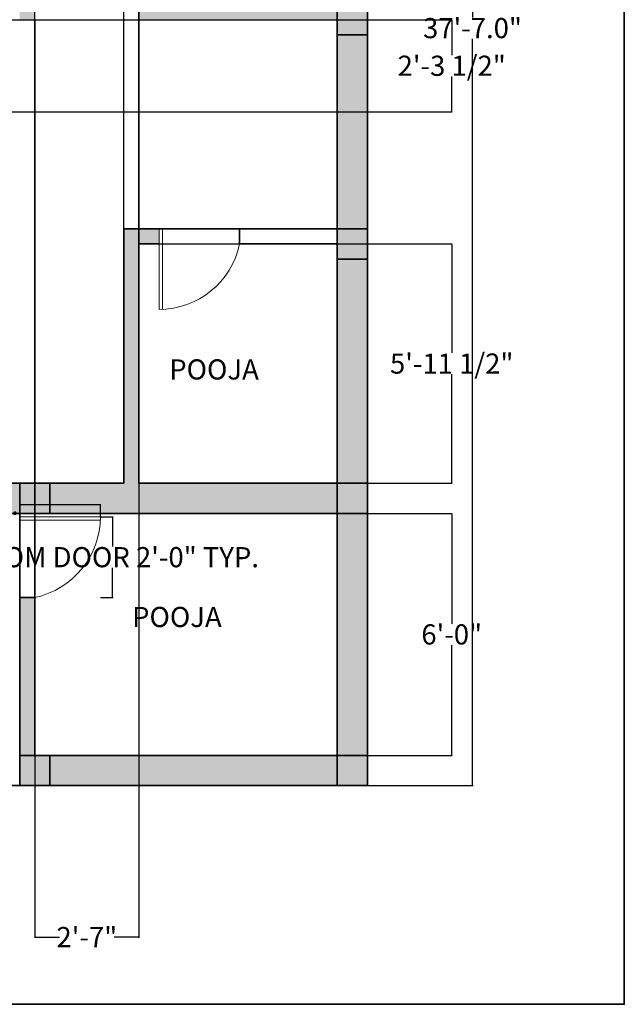
# Model space of a CAD drawing. Units: inches. Extents: x 74 to 548, y 68 to 649.
# Tile 3 of 6: x 368 to 548, y 68 to 361. Entities that reach past the tile are written whole.
import ezdxf

# ---------------------------------------------------------------- set-up
doc = ezdxf.new("R2010")
doc.units = ezdxf.units.IN
doc.header["$MEASUREMENT"] = 0
for name, color, linetype, lineweight in [('A-ANNO-DIMS', 2, 'Continuous', 18), ('A-ANNO-TTLB', 7, 'Continuous', 35), ('A-AREA-IDEN', 7, 'Continuous', 25), ('A-COLS', 7, 'Continuous', 35), ('A-DOOR', 3, 'Continuous', 18), ('A-WALL', 7, 'Continuous', 35)]:
    doc.layers.add(name, color=color, linetype=linetype, lineweight=lineweight)
doc.layers.add('A-COLS-PATT', color=11, linetype='Continuous', lineweight=13, true_color=0xf27172)
doc.layers.add('A-WALL-PATT', color=7, linetype='Continuous', lineweight=13, true_color=0xffffff)
doc.styles.get("Standard").update_dxf_attribs({"font": 'arial.ttf'})
doc.dimstyles.get("Standard").update_dxf_attribs({"dimtxt": 6, "dimasz": 0.18, "dimexe": 0.18, "dimexo": 0.0625, "dimgap": 0.09, "dimtad": 0, "dimtih": 1, "dimtoh": 1, "dimdec": 1, "dimzin": 0, "dimdsep": 46, "dimlunit": 3, "dimtxsty": 'Standard', "dimcen": 0.09, "dimadec": 0, "dimazin": 0, "dimtfac": 1, "dimtdec": 1, "dimtofl": 0, "dimtmove": 0, "dimatfit": 3, "dimfxl": 1, "dimtolj": 1, "dimtzin": 0, "dimarcsym": 0})

# ---------------------------------------------------------------- blocks, each defined once
blk = doc.blocks.new('*D4')
at = {"layer": 'A-ANNO-DIMS', "color": 0, "lineweight": -2, "transparency": 16777216}
for p, q in [((472.02, 584.24), (503.43, 584.24)), ((503.25, 584.06), (503.25, 361.9)), ((503.25, 133.42), (503.25, 355.59)), ((472.02, 133.24), (503.43, 133.24))]:
    blk.add_line(p, q, dxfattribs=at)
at = {"layer": 'A-ANNO-DIMS', "color": 0, "transparency": 16777216}
for points in [[(503.22, 584.06), (503.28, 584.06), (503.25, 584.24)], [(503.22, 133.42), (503.28, 133.42), (503.25, 133.24)]]:
    blk.add_solid(points, dxfattribs=at)
at = {"layer": 'Defpoints', "color": 0, "transparency": 16777216}
for p in [(471.96, 584.24), (471.96, 133.24), (503.25, 133.24)]:
    blk.add_point(p, dxfattribs=at)
at = {"layer": 'A-ANNO-DIMS', "color": 0, "transparency": 16777216, "insert": (503.25, 358.74), "char_height": 6, "attachment_point": 5}
blk.add_mtext('\\A1;37\'-7.0"', dxfattribs=at)
blk = doc.blocks.new('DOOR-SWING-24IN')
for p, q in [((0, 0), (-24, 0)), ((-1, -24), (-1, 0)), ((0, 0), (0, -24))]:
    blk.add_line(p, q)
blk.add_arc((0, 0.52), 24.52, 191.8123, 270)
blk = doc.blocks.new('*D16')
at = {"layer": 'A-ANNO-DIMS', "color": 0, "lineweight": -2, "transparency": 16777216}
for p, q in [((392.52, 213.24), (396.24, 213.24)), ((396.06, 213.06), (396.06, 204.44)), ((396.06, 189.42), (396.06, 198.05)), ((392.52, 189.24), (396.24, 189.24))]:
    blk.add_line(p, q, dxfattribs=at)
at = {"layer": 'A-ANNO-DIMS', "color": 0, "transparency": 16777216}
for points in [[(396.03, 213.06), (396.09, 213.06), (396.06, 213.24)], [(396.03, 189.42), (396.09, 189.42), (396.06, 189.24)]]:
    blk.add_solid(points, dxfattribs=at)
at = {"layer": 'Defpoints', "color": 0, "transparency": 16777216}
for p in [(392.46, 213.24), (396.06, 213.24), (392.46, 189.24)]:
    blk.add_point(p, dxfattribs=at)
at = {"layer": 'A-ANNO-DIMS', "color": 0, "transparency": 16777216, "insert": (396.06, 201.24), "char_height": 6, "attachment_point": 5}
blk.add_mtext('\\A1;ROOM DOOR 2\'-0" TYP.', dxfattribs=at)
blk = doc.blocks.new('*D17')
at = {"layer": 'A-ANNO-DIMS', "color": 0, "lineweight": -2, "transparency": 16777216}
for p, q in [((368.46, 213.31), (368.46, 217.02)), ((392.46, 213.31), (392.46, 217.02)), ((368.46, 216.84), (368.28, 216.84)), ((392.28, 216.84), (368.64, 216.84))]:
    blk.add_line(p, q, dxfattribs=at)
at = {"layer": 'A-ANNO-DIMS', "color": 0, "transparency": 16777216}
for points in [[(368.64, 216.87), (368.64, 216.81), (368.46, 216.84)], [(392.28, 216.87), (392.28, 216.81), (392.46, 216.84)]]:
    blk.add_solid(points, dxfattribs=at)
at = {"layer": 'Defpoints', "color": 0, "transparency": 16777216}
for p in [(368.46, 216.84), (368.46, 213.24), (392.46, 213.24)]:
    blk.add_point(p, dxfattribs=at)
at = {"layer": 'A-ANNO-DIMS', "color": 0, "transparency": 16777216, "insert": (349.85, 216.84), "char_height": 6, "attachment_point": 5}
blk.add_mtext('\\A1;2\'-0" TYP.', dxfattribs=at)
blk = doc.blocks.new('*D21')
at = {"layer": 'A-ANNO-DIMS', "color": 0, "lineweight": -2, "transparency": 16777216}
for p, q in [((372.96, 361.31), (372.96, 609.52)), ((373.14, 609.34), (409.92, 609.34)), ((462.78, 609.34), (426, 609.34)), ((462.96, 356.81), (462.96, 609.52))]:
    blk.add_line(p, q, dxfattribs=at)
at = {"layer": 'A-ANNO-DIMS', "color": 0, "transparency": 16777216}
for points in [[(373.14, 609.37), (373.14, 609.31), (372.96, 609.34)], [(462.78, 609.37), (462.78, 609.31), (462.96, 609.34)]]:
    blk.add_solid(points, dxfattribs=at)
at = {"layer": 'Defpoints', "color": 0, "transparency": 16777216}
for p in [(462.96, 609.34), (372.96, 361.24), (462.96, 356.74)]:
    blk.add_point(p, dxfattribs=at)
at = {"layer": 'A-ANNO-DIMS', "color": 0, "transparency": 16777216, "insert": (417.96, 609.34), "char_height": 6, "attachment_point": 5}
blk.add_mtext('\\A1;7\'-6"', dxfattribs=at)
blk = doc.blocks.new('*D24')
at = {"layer": 'A-ANNO-DIMS', "color": 0, "lineweight": -2, "transparency": 16777216}
for p, q in [((403.93, 223.31), (403.93, 609.52)), ((404.11, 609.34), (422.93, 609.34)), ((462.78, 609.34), (443.96, 609.34)), ((462.96, 133.31), (462.96, 609.52))]:
    blk.add_line(p, q, dxfattribs=at)
at = {"layer": 'A-ANNO-DIMS', "color": 0, "transparency": 16777216}
for points in [[(404.11, 609.37), (404.11, 609.31), (403.93, 609.34)], [(462.78, 609.37), (462.78, 609.31), (462.96, 609.34)]]:
    blk.add_solid(points, dxfattribs=at)
at = {"layer": 'Defpoints', "color": 0, "transparency": 16777216}
for p in [(462.96, 609.34), (403.93, 223.24), (462.96, 133.24)]:
    blk.add_point(p, dxfattribs=at)
at = {"layer": 'A-ANNO-DIMS', "color": 0, "transparency": 16777216, "insert": (433.44, 609.34), "char_height": 6, "attachment_point": 5}
blk.add_mtext('\\A1;4\'-11"', dxfattribs=at)
blk = doc.blocks.new('*D25')
at = {"layer": 'A-ANNO-DIMS', "color": 0, "lineweight": -2, "transparency": 16777216}
for p, q in [((403.99, 294.49), (497.24, 294.49)), ((497.06, 294.31), (497.06, 262.06)), ((497.06, 223.42), (497.06, 255.68)), ((403.99, 223.24), (497.24, 223.24))]:
    blk.add_line(p, q, dxfattribs=at)
at = {"layer": 'A-ANNO-DIMS', "color": 0, "transparency": 16777216}
for points in [[(497.03, 294.31), (497.09, 294.31), (497.06, 294.49)], [(497.03, 223.42), (497.09, 223.42), (497.06, 223.24)]]:
    blk.add_solid(points, dxfattribs=at)
at = {"layer": 'Defpoints', "color": 0, "transparency": 16777216}
for p in [(403.93, 294.49), (497.06, 294.49), (403.93, 223.24)]:
    blk.add_point(p, dxfattribs=at)
at = {"layer": 'A-ANNO-DIMS', "color": 0, "transparency": 16777216, "insert": (497.06, 258.87), "char_height": 6, "attachment_point": 5}
blk.add_mtext('\\A1;5\'-11 1/2"', dxfattribs=at)
blk = doc.blocks.new('*D26')
at = {"layer": 'A-ANNO-DIMS', "color": 0, "lineweight": -2, "transparency": 16777216}
for p, q in [((372.96, 142.31), (372.96, 609.52)), ((373.14, 609.34), (409.92, 609.34)), ((462.78, 609.34), (426, 609.34)), ((462.96, 133.31), (462.96, 609.52))]:
    blk.add_line(p, q, dxfattribs=at)
at = {"layer": 'A-ANNO-DIMS', "color": 0, "transparency": 16777216}
for points in [[(373.14, 609.37), (373.14, 609.31), (372.96, 609.34)], [(462.78, 609.37), (462.78, 609.31), (462.96, 609.34)]]:
    blk.add_solid(points, dxfattribs=at)
at = {"layer": 'Defpoints', "color": 0, "transparency": 16777216}
for p in [(462.96, 609.34), (372.96, 142.24), (462.96, 133.24)]:
    blk.add_point(p, dxfattribs=at)
at = {"layer": 'A-ANNO-DIMS', "color": 0, "transparency": 16777216, "insert": (417.96, 609.34), "char_height": 6, "attachment_point": 5}
blk.add_mtext('\\A1;7\'-6"', dxfattribs=at)
blk = doc.blocks.new('*D27')
at = {"layer": 'A-ANNO-DIMS', "color": 0, "lineweight": -2, "transparency": 16777216}
for p, q in [((377.52, 214.24), (497.24, 214.24)), ((497.06, 214.06), (497.06, 181.4)), ((497.06, 142.42), (497.06, 175.09)), ((373.02, 142.24), (497.24, 142.24))]:
    blk.add_line(p, q, dxfattribs=at)
at = {"layer": 'A-ANNO-DIMS', "color": 0, "transparency": 16777216}
for points in [[(497.03, 214.06), (497.09, 214.06), (497.06, 214.24)], [(497.03, 142.42), (497.09, 142.42), (497.06, 142.24)]]:
    blk.add_solid(points, dxfattribs=at)
at = {"layer": 'Defpoints', "color": 0, "transparency": 16777216}
for p in [(377.46, 214.24), (497.06, 214.24), (372.96, 142.24)]:
    blk.add_point(p, dxfattribs=at)
at = {"layer": 'A-ANNO-DIMS', "color": 0, "transparency": 16777216, "insert": (497.06, 178.24), "char_height": 6, "attachment_point": 5}
blk.add_mtext('\\A1;6\'-0"', dxfattribs=at)
blk = doc.blocks.new('*D37')
at = {"layer": 'A-ANNO-DIMS', "color": 0, "lineweight": -2, "transparency": 16777216}
for p, q in [((266.46, 297.87), (266.46, 609.52)), ((266.64, 609.34), (322.83, 609.34)), ((399.25, 609.34), (343.06, 609.34)), ((399.43, 299.06), (399.43, 609.52))]:
    blk.add_line(p, q, dxfattribs=at)
at = {"layer": 'A-ANNO-DIMS', "color": 0, "transparency": 16777216}
for points in [[(266.64, 609.37), (266.64, 609.31), (266.46, 609.34)], [(399.25, 609.37), (399.25, 609.31), (399.43, 609.34)]]:
    blk.add_solid(points, dxfattribs=at)
at = {"layer": 'Defpoints', "color": 0, "transparency": 16777216}
for p in [(399.43, 609.34), (399.43, 298.99), (266.46, 297.81)]:
    blk.add_point(p, dxfattribs=at)
at = {"layer": 'A-ANNO-DIMS', "color": 0, "transparency": 16777216, "insert": (332.94, 609.34), "char_height": 6, "attachment_point": 5}
blk.add_mtext('\\A1;11\'-1"', dxfattribs=at)
blk = doc.blocks.new('*D39')
at = {"layer": 'A-ANNO-DIMS', "color": 0, "lineweight": -2, "transparency": 16777216}
for p, q in [((403.93, 365.68), (403.93, 87.96)), ((372.96, 361.18), (372.96, 87.96)), ((373.14, 88.14), (380.33, 88.14)), ((403.75, 88.14), (396.56, 88.14))]:
    blk.add_line(p, q, dxfattribs=at)
at = {"layer": 'A-ANNO-DIMS', "color": 0, "transparency": 16777216}
for points in [[(373.14, 88.17), (373.14, 88.11), (372.96, 88.14)], [(403.75, 88.17), (403.75, 88.11), (403.93, 88.14)]]:
    blk.add_solid(points, dxfattribs=at)
at = {"layer": 'Defpoints', "color": 0, "transparency": 16777216}
for p in [(403.93, 365.74), (372.96, 361.24), (403.93, 88.14)]:
    blk.add_point(p, dxfattribs=at)
at = {"layer": 'A-ANNO-DIMS', "color": 0, "transparency": 16777216, "insert": (388.44, 88.14), "char_height": 6, "attachment_point": 5}
blk.add_mtext('\\A1;2\'-7"', dxfattribs=at)
blk = doc.blocks.new('*D41')
at = {"layer": 'A-ANNO-DIMS', "color": 0, "lineweight": -2, "transparency": 16777216}
for p, q in [((257.52, 361.24), (497.24, 361.24)), ((497.06, 361.06), (497.06, 350.72)), ((497.06, 333.99), (497.06, 344.33)), ((262.02, 333.81), (497.24, 333.81))]:
    blk.add_line(p, q, dxfattribs=at)
at = {"layer": 'A-ANNO-DIMS', "color": 0, "transparency": 16777216}
for points in [[(497.03, 361.06), (497.09, 361.06), (497.06, 361.24)], [(497.03, 333.99), (497.09, 333.99), (497.06, 333.81)]]:
    blk.add_solid(points, dxfattribs=at)
at = {"layer": 'Defpoints', "color": 0, "transparency": 16777216}
for p in [(257.46, 361.24), (497.06, 361.24), (261.96, 333.81)]:
    blk.add_point(p, dxfattribs=at)
at = {"layer": 'A-ANNO-DIMS', "color": 0, "transparency": 16777216, "insert": (497.06, 347.53), "char_height": 6, "attachment_point": 5}
blk.add_mtext('\\A1;2\'-3 1/2"', dxfattribs=at)

msp = doc.modelspace()

# ---------------------------------------------------------------- hatches: boundary and pattern name
at = {"layer": 'A-COLS-PATT'}
h = msp.add_hatch(color=256, dxfattribs=at)
h.dxf.hatch_style = 1
h.paths.add_polyline_path([(123.96, 584.24), (114.96, 584.24), (114.96, 575.24), (123.96, 575.24)])
h.paths.add_polyline_path([(266.46, 584.24), (257.46, 584.24), (257.46, 575.24), (266.46, 575.24)])
h.paths.add_polyline_path([(329.46, 584.24), (320.46, 584.24), (320.46, 575.24), (329.46, 575.24)])
h.paths.add_polyline_path([(471.96, 584.24), (462.96, 584.24), (462.96, 575.24), (471.96, 575.24)])
h.paths.add_polyline_path([(123.96, 448.24), (114.96, 448.24), (114.96, 439.24), (123.96, 439.24)])
h.paths.add_polyline_path([(266.46, 448.24), (261.96, 448.24), (257.46, 448.24), (257.46, 439.24), (266.46, 439.24)])
h.paths.add_polyline_path([(329.46, 448.24), (320.46, 448.24), (320.46, 439.24), (329.46, 439.24)])
h.paths.add_polyline_path([(471.96, 448.24), (462.96, 448.24), (462.96, 439.24), (471.96, 439.24)])
h.paths.add_polyline_path([(123.96, 365.74), (114.96, 365.74), (114.96, 356.74), (123.96, 356.74)])
h.paths.add_polyline_path([(266.46, 365.74), (257.46, 365.74), (257.46, 356.74), (266.46, 356.74)])
h.paths.add_polyline_path([(123.96, 223.24), (114.96, 223.24), (114.96, 214.24), (123.96, 214.24)])
h.paths.add_polyline_path([(266.46, 223.24), (257.46, 223.24), (257.46, 214.24), (266.46, 214.24)])
h.paths.add_polyline_path([(123.96, 142.24), (114.96, 142.24), (114.96, 133.24), (123.96, 133.24)])
h.paths.add_polyline_path([(263.89, 142.24), (254.89, 142.24), (254.89, 133.24), (263.89, 133.24)])
h.paths.add_polyline_path([(471.96, 142.24), (462.96, 142.24), (462.96, 133.24), (471.96, 133.24)])
h.paths.add_polyline_path([(377.46, 142.24), (368.46, 142.24), (368.46, 133.24), (377.46, 133.24)])
h.paths.add_polyline_path([(377.46, 223.24), (368.46, 223.24), (368.46, 214.24), (377.46, 214.24)])
h.paths.add_polyline_path([(471.96, 223.24), (462.96, 223.24), (462.96, 214.24), (471.96, 214.24)])
h.paths.add_polyline_path([(471.96, 298.99), (462.96, 298.99), (462.96, 289.99), (471.96, 289.99)])
h.paths.add_polyline_path([(471.96, 365.74), (462.96, 365.74), (462.96, 356.74), (471.96, 356.74)])
at = {"layer": 'A-WALL-PATT'}
h = msp.add_hatch(color=256, dxfattribs=at)
h.dxf.hatch_style = 1
h.paths.add_polyline_path([(123.96, 356.74), (114.96, 356.74), (114.96, 223.24), (123.96, 223.24)])
h.paths.add_polyline_path([(123.96, 439.24), (114.96, 439.24), (114.96, 365.74), (123.96, 365.74)])
h.paths.add_polyline_path([(123.96, 575.24), (114.96, 575.24), (114.96, 448.24), (123.96, 448.24)])
h.paths.add_polyline_path([(257.46, 584.24), (123.96, 584.24), (123.96, 575.24), (257.46, 575.24)])
h.paths.add_polyline_path([(266.46, 575.24), (261.96, 575.24), (261.96, 490.24), (266.46, 490.24)])
h.paths.add_polyline_path([(266.46, 454.24), (261.96, 454.24), (261.96, 448.24), (266.46, 448.24)])
h.paths.add_polyline_path([(257.46, 448.24), (187.71, 448.24), (187.71, 443.74), (190.71, 443.74), (190.71, 365.74), (123.96, 365.74), (123.96, 361.24), (257.46, 361.24), (257.46, 365.74), (195.21, 365.74), (195.21, 443.74), (257.46, 443.74)])
h.paths.add_polyline_path([(163.71, 448.24), (123.96, 448.24), (123.96, 443.74), (163.71, 443.74)], flags=17)
h.paths.add_polyline_path([(223.59, 223.24), (220.05, 223.24), (220.05, 216.24), (160.05, 216.24), (160.05, 223.24), (123.96, 223.24), (123.96, 214.24), (159.96, 214.24), (223.59, 214.24)])
h.paths.add_polyline_path([(123.96, 214.24), (114.96, 214.24), (114.96, 142.24), (123.96, 142.24)])
h.paths.add_polyline_path([(254.89, 142.24), (123.96, 142.24), (123.96, 133.24), (254.89, 133.24)])
h.paths.add_polyline_path([(462.96, 142.24), (377.46, 142.24), (377.46, 133.24), (462.96, 133.24)])
h.paths.add_polyline_path([(372.96, 189.24), (368.46, 189.24), (368.46, 142.24), (372.96, 142.24)])
h.paths.add_polyline_path([(471.96, 214.24), (462.96, 214.24), (462.96, 142.24), (471.96, 142.24)])
h.paths.add_polyline_path([(462.96, 223.24), (403.93, 223.24), (403.93, 294.49), (409.93, 294.49), (409.93, 298.99), (403.93, 298.99), (399.43, 298.99), (399.43, 223.24), (377.46, 223.24), (377.46, 214.24), (462.96, 214.24)])
h.paths.add_polyline_path([(368.46, 223.24), (353.46, 223.24), (353.46, 216.24), (305.46, 216.24), (305.46, 223.24), (302.46, 223.24), (302.46, 214.24), (368.46, 214.24)])
h.paths.add_polyline_path([(471.96, 289.99), (462.96, 289.99), (462.96, 223.24), (471.96, 223.24)])
h.paths.add_polyline_path([(462.96, 298.99), (433.93, 298.99), (433.93, 294.49), (462.96, 294.49)], flags=0)
h.paths.add_polyline_path([(471.96, 356.74), (462.96, 356.74), (462.96, 298.99), (471.96, 298.99)])
h.paths.add_polyline_path([(462.96, 365.74), (403.93, 365.74), (403.93, 361.24), (462.96, 361.24)], flags=17)
h.paths.add_polyline_path([(471.96, 439.24), (462.96, 439.24), (462.96, 365.74), (471.96, 365.74)])
h.paths.add_polyline_path([(462.96, 448.24), (329.46, 448.24), (329.46, 439.24), (368.46, 439.24), (368.46, 361.24), (372.96, 361.24), (372.96, 443.74), (462.96, 443.74)])
h.paths.add_polyline_path([(324.96, 454.24), (320.46, 454.24), (320.46, 448.24), (324.96, 448.24)])
h.paths.add_polyline_path([(471.96, 575.24), (462.96, 575.24), (462.96, 448.24), (471.96, 448.24)])
h.paths.add_polyline_path([(462.96, 584.24), (329.46, 584.24), (329.46, 575.24), (462.96, 575.24)])
h.paths.add_polyline_path([(320.46, 584.24), (266.46, 584.24), (266.46, 575.24), (320.46, 575.24)])
h.paths.add_polyline_path([(324.96, 575.24), (320.46, 575.24), (320.46, 490.24), (324.96, 490.24)])
h.paths.add_polyline_path([(266.46, 405.58), (257.46, 405.58), (257.46, 365.74), (266.46, 365.74)])
h.paths.add_polyline_path([(266.46, 356.74), (261.96, 356.74), (261.96, 333.81), (266.46, 333.81)])
h.paths.add_polyline_path([(266.46, 297.81), (261.96, 297.81), (261.96, 223.24), (266.46, 223.24)])

# ---------------------------------------------------------------- linework, layer by layer
at = {"layer": 'A-ANNO-TTLB'}
msp.add_lwpolyline([(82.75, 649.38), (548.44, 649.38), (548.44, 68.13), (82.75, 68.13)], close=True, dxfattribs=at)
at = {"layer": 'A-COLS'}
for p, q in [((471.96, 356.74), (462.96, 356.74)), ((471.96, 289.99), (462.96, 289.99)), ((377.46, 223.24), (377.46, 214.24)), ((368.46, 142.24), (377.46, 142.24)), ((377.46, 142.24), (377.46, 133.24)), ((377.46, 133.24), (368.46, 133.24))]:
    msp.add_line(p, q, dxfattribs=at)
at = {"layer": 'A-DOOR'}
for p, q in [((409.93, 274.99), (409.93, 298.99)), ((392.46, 213.24), (368.46, 213.24))]:
    msp.add_line(p, q, dxfattribs=at)
at = {"layer": 'A-WALL'}
for p, q in [((462.96, 584.24), (462.96, 133.24)), ((471.96, 584.24), (471.96, 133.24)), ((399.43, 298.99), (471.96, 298.99)), ((399.43, 223.24), (399.43, 298.99)), ((403.93, 298.99), (409.93, 298.99)), ((433.93, 298.99), (433.93, 294.49)), ((403.93, 223.24), (403.93, 294.49)), ((403.93, 294.49), (409.93, 294.49)), ((433.93, 294.49), (462.96, 294.49)), ((302.46, 223.24), (399.43, 223.24)), ((368.46, 223.24), (368.46, 133.24)), ((403.93, 223.24), (471.96, 223.24)), ((114.96, 214.24), (471.96, 214.24)), ((368.46, 214.24), (368.46, 213.24)), ((372.96, 214.24), (372.96, 213.24)), ((368.46, 189.24), (372.96, 189.24)), ((372.96, 189.24), (372.96, 142.24)), ((368.46, 142.24), (471.96, 142.24)), ((114.96, 133.24), (471.96, 133.24))]:
    msp.add_line(p, q, dxfattribs=at)

# ---------------------------------------------------------------- block references
at = {"layer": 'A-DOOR', "extrusion": (0, 0, -1), "zscale": -1}
msp.add_blockref('DOOR-SWING-24IN', (-409.93, 298.99), dxfattribs=at)
at = {"layer": 'A-DOOR', "rotation": 89.99999999999996}
msp.add_blockref('DOOR-SWING-24IN', (368.46, 213.24), dxfattribs=at)

# ---------------------------------------------------------------- texts
at = {"layer": 'A-AREA-IDEN', "char_height": 6, "attachment_point": 1}
for width, insert in [(37.4475, (412.96, 260.13)), (46.0396, (401.91, 186.44))]:
    msp.add_mtext_dynamic_manual_height_columns('POOJA', width=width, gutter_width=30, heights=[0], dxfattribs=dict(at, insert=insert))

# ---------------------------------------------------------------- dimensions: what is measured, and where the dimension line sits
at = {"layer": 'A-ANNO-DIMS'}
for base, p1, p2, picture, middle in [((399.43, 609.34), (266.46, 297.81), (399.43, 298.99), '*D37', (332.94, 609.34)), ((462.96, 609.34), (372.96, 361.24), (462.96, 356.74), '*D21', (417.96, 609.34)), ((462.96, 609.34), (372.96, 142.24), (462.96, 133.24), '*D26', (417.96, 609.34)), ((462.96, 609.34), (403.93, 223.24), (462.96, 133.24), '*D24', (433.44, 609.34)), ((403.93, 88.14), (372.96, 361.24), (403.93, 365.74), '*D39', (388.44, 88.14))]:
    dim = msp.add_linear_dim(base=base, p1=p1, p2=p2, dimstyle='Standard', override={"dimdec": 1, "dimlfac": 1, "dimrnd": 0, "dimzin": 1, "dimdsep": 46, "dimlunit": 4, "dimfrac": 2}, dxfattribs=at)
    dim.commit()
    dim.dimension.update_dxf_attribs({"geometry": picture, "text_midpoint": middle})
for base, p1, p2, override, picture, middle in [((503.25, 133.24), (471.96, 584.24), (471.96, 133.24), {"dimclrd": 0, "dimclre": 0, "dimclrt": 0}, '*D4', (503.25, 358.74)), ((497.06, 361.24), (261.96, 333.81), (257.46, 361.24), {"dimdec": 1, "dimlfac": 1, "dimrnd": 0, "dimzin": 1, "dimdsep": 46, "dimlunit": 4, "dimfrac": 2}, '*D41', (497.06, 347.53)), ((497.060646, 294.492592), (403.926686, 223.242592), (403.926686, 294.492592), {"dimdec": 1, "dimlfac": 1, "dimrnd": 0, "dimzin": 1, "dimdsep": 46, "dimlunit": 4, "dimfrac": 2}, '*D25', (497.060646, 258.867592)), ((497.06, 214.24), (372.96, 142.24), (377.46, 214.24), {"dimdec": 1, "dimlfac": 1, "dimrnd": 0, "dimzin": 1, "dimdsep": 46, "dimlunit": 4, "dimfrac": 2}, '*D27', (497.06, 178.24))]:
    dim = msp.add_linear_dim(base=base, p1=p1, p2=p2, angle=90, dimstyle='Standard', override=override, dxfattribs=at)
    dim.commit()
    dim.dimension.update_dxf_attribs({"geometry": picture, "text_midpoint": middle})
for base, p1, p2, angle, text, picture, middle in [((368.46, 216.84), (392.46, 213.24), (368.46, 213.24), 180, '<> TYP.', '*D17', (349.85, 216.84)), ((396.06, 213.24), (392.46, 189.24), (392.46, 213.24), 90, 'ROOM DOOR <> TYP.', '*D16', (396.06, 201.24))]:
    dim = msp.add_linear_dim(base=base, p1=p1, p2=p2, angle=angle, text=text, dimstyle='Standard', override={"dimdec": 1, "dimlfac": 1, "dimrnd": 0, "dimzin": 1, "dimdsep": 46, "dimlunit": 4, "dimfrac": 2}, dxfattribs=at)
    dim.commit()
    dim.dimension.update_dxf_attribs({"geometry": picture, "text_midpoint": middle})

doc.saveas('drawing.dxf')
